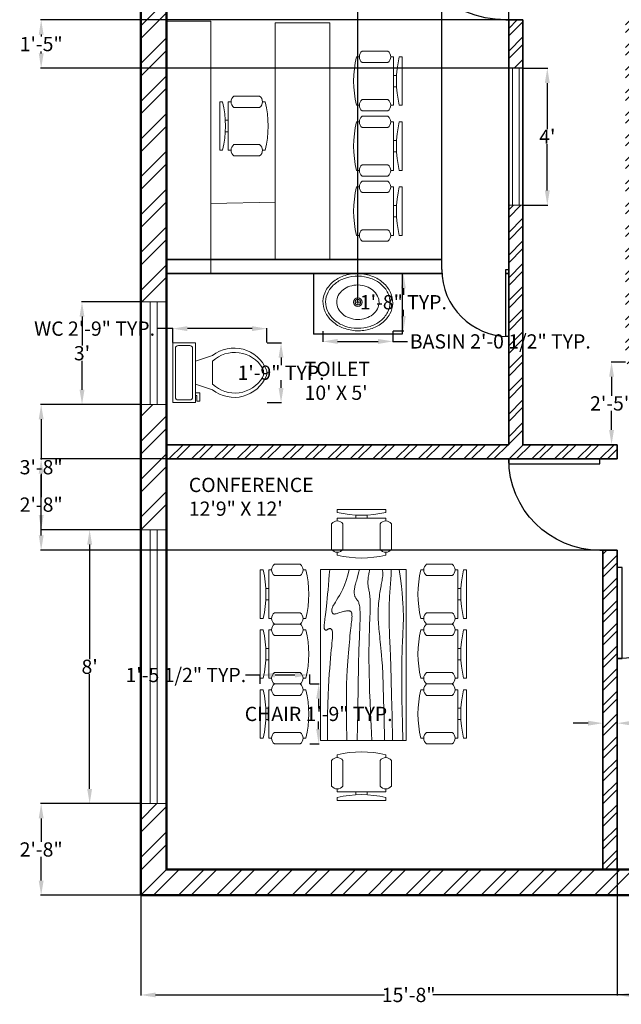
# Model space of a CAD drawing. Units: inches. Extents: x -355 to 263, y -871 to -163.
# Tile 1 of 6: x -344 to -133, y -867 to -521. Entities that reach past the tile are written whole.
import ezdxf

# ---------------------------------------------------------------- set-up
doc = ezdxf.new("R2010")
doc.units = ezdxf.units.IN
doc.header["$MEASUREMENT"] = 0
doc.layers.get('Defpoints').update_dxf_attribs({"color": 50})
for name, color, linetype, lineweight in [('A-ANNO-DIMS', 2, 'Continuous', 18), ('A-AREA-IDEN', 7, 'Continuous', 18), ('A-FLOR-CASE', 9, 'Continuous', 25), ('A-FLOR-FIXT', 8, 'Continuous', 18), ('A-WALL-PATT', 252, 'Continuous', 13)]:
    doc.layers.add(name, color=color, linetype=linetype, lineweight=lineweight)
for name, color, linetype, lineweight, plot in [('CHAIR', 8, 'Continuous', 18, False), ('DOOR', 4, 'Continuous', 25, False), ('IWAL', 7, 'Continuous', 35, False), ('OWALL', 7, 'Continuous', 50, False), ('TABLE', 8, 'Continuous', 18, False), ('WIND', 3, 'Continuous', 18, False)]:
    doc.layers.add(name, color=color, linetype=linetype, lineweight=lineweight, plot=plot)
doc.styles.get("Standard").update_dxf_attribs({"font": 'arial.ttf'})
doc.dimstyles.get("Standard").update_dxf_attribs({"dimtxt": 5, "dimasz": 5.18, "dimexe": 0.18, "dimexo": 0.0625, "dimgap": 0.09, "dimtad": 0, "dimtih": 1, "dimtoh": 1, "dimdec": 0, "dimzin": 0, "dimdsep": 46, "dimlunit": 3, "dimtxsty": 'Standard', "dimcen": 0.09, "dimadec": 0, "dimazin": 0, "dimtfac": 1, "dimtdec": 0, "dimtofl": 0, "dimtmove": 0, "dimatfit": 3, "dimfxl": 1, "dimtolj": 1, "dimtzin": 0, "dimarcsym": 0})

# ---------------------------------------------------------------- blocks, each defined once
blk = doc.blocks.new('*U6')
for p, q in [((0, 0), (0, -6)), ((32, 0), (32, -6))]:
    blk.add_line(p, q)
blk.add_lwpolyline([(0, 0), (0, 32), (1.75, 32), (1.75, 0)], close=True)
blk.add_arc((0, 0), 32, 0, 90)
blk = doc.blocks.new('*U5')
for p, q in [((0, 0), (0, -6)), ((40, 0), (40, -6))]:
    blk.add_line(p, q)
blk.add_lwpolyline([(0, 0), (0, 40), (1.75, 40), (1.75, 0)], close=True)
blk.add_arc((0, 0), 40, 0, 90)
blk = doc.blocks.new('*U7')
for p, q in [((0, 0), (0, -6)), ((36, 0), (36, -6))]:
    blk.add_line(p, q)
blk.add_lwpolyline([(0, 0), (0, 36), (1.75, 36), (1.75, 0)], close=True)
blk.add_arc((0, 0), 36, 0, 90)
blk = doc.blocks.new('Table - Rectangular Woodgrain 60 x 30 in.')
for p, q in [((0, 0), (0, -30)), ((60, 0), (0, 0)), ((60, -30), (60, 0)), ((0, -30), (60, -30))]:
    blk.add_line(p, q)
for points in [[(0, -2.4), (4.8155, -2.418), (9.0302, -2.4688), (12.709, -2.5477), (15.9167, -2.65), (18.7181, -2.7711), (21.1781, -2.9063), (23.3616, -3.0508), (25.3333, -3.2), (27.1477, -3.3495), (28.8172, -3.4958), (30.3437, -3.636), (31.7291, -3.7667), (32.9756, -3.8849), (34.0849, -3.9875), (35.059, -4.0714), (35.9, -4.1334), (36.6114, -4.1711), (37.2041, -4.1854), (37.6906, -4.1779), (38.0833, -4.15), (38.3948, -4.1034), (38.6375, -4.0396), (38.8239, -3.9602), (38.9666, -3.8667), (39.0764, -3.7608), (39.1573, -3.6448), (39.2116, -3.521), (39.2416, -3.3917), (39.2498, -3.2593), (39.2385, -3.1261), (39.21, -2.9944), (39.1666, -2.8667), (39.111, -2.7447), (39.0468, -2.6281), (38.978, -2.5163), (38.9083, -2.4083), (38.8418, -2.3035), (38.7823, -2.201), (38.7337, -2.1001), (38.7, -2), (38.6844, -1.9003), (38.6875, -1.8021), (38.7094, -1.707), (38.75, -1.6167), (38.8094, -1.5326), (38.8875, -1.4563), (38.9844, -1.3893), (39.1, -1.3333), (39.2351, -1.2896), (39.3937, -1.2583), (39.5804, -1.2396), (39.8, -1.2333), (40.057, -1.2396), (40.3562, -1.2583), (40.7023, -1.2896), (41.1, -1.3333), (41.5547, -1.3895), (42.0755, -1.4573), (42.6721, -1.5361), (43.3542, -1.625), (44.1316, -1.7233), (45.014, -1.8302), (46.0114, -1.9449), (47.1333, -2.0667), (48.3862, -2.1947), (49.7625, -2.3281), (51.2513, -2.4663), (52.8416, -2.6083), (54.5226, -2.7535), (56.2833, -2.9011), (58.1127, -3.0501), (60, -3.2)], [(0, -9.2), (6.5759, -9.0858), (11.9385, -9.0365), (16.2527, -9.0418), (19.6833, -9.0917), (22.3952, -9.1759), (24.5531, -9.2844), (26.322, -9.4069), (27.8666, -9.5333), (29.3241, -9.6553), (30.7203, -9.7719), (32.0532, -9.8837), (33.3208, -9.9917), (34.5213, -10.0965), (35.6526, -10.199), (36.7128, -10.2999), (37.7, -10.4), (38.6129, -10.4996), (39.4531, -10.5969), (40.223, -10.6895), (40.925, -10.775), (41.5613, -10.8512), (42.1344, -10.9156), (42.6465, -10.966), (43.1, -11), (43.4976, -11.0158), (43.8437, -11.0136), (44.143, -10.9942), (44.4, -10.9583), (44.6195, -10.9069), (44.8062, -10.8406), (44.9648, -10.7603), (45.1, -10.6667), (45.2155, -10.5598), (45.3114, -10.4365), (45.3871, -10.2929), (45.4416, -10.125), (45.4743, -9.929), (45.4844, -9.7011), (45.4709, -9.4371), (45.4333, -9.1333), (45.3716, -8.7883), (45.2896, -8.4104), (45.1919, -8.0107), (45.0833, -7.6), (44.9685, -7.1893), (44.8521, -6.7896), (44.7388, -6.4117), (44.6333, -6.0667), (44.54, -5.7628), (44.4614, -5.4979), (44.4001, -5.2675), (44.3583, -5.0667), (44.3384, -4.8909), (44.3427, -4.7354), (44.3736, -4.5956), (44.4333, -4.4667), (44.5236, -4.3453), (44.6427, -4.2333), (44.7884, -4.1339), (44.9583, -4.05), (45.1501, -3.9849), (45.3614, -3.9417), (45.59, -3.9234), (45.8333, -3.9333), (46.0915, -3.9749), (46.3734, -4.0531), (46.6906, -4.1736), (47.0542, -4.3417), (47.4756, -4.5629), (47.9661, -4.8427), (48.5372, -5.1866), (49.2, -5.6), (49.9676, -6.0844), (50.8594, -6.625), (51.8965, -7.2031), (53.1, -7.8), (54.491, -8.3969), (56.0906, -8.975), (57.9199, -9.5156), (60, -10)], [(0, -12.8), (5.1847, -12.9322), (9.6213, -13.0323), (13.3963, -13.1059), (16.5958, -13.1583), (19.3063, -13.1952), (21.614, -13.2219), (23.6054, -13.2439), (25.3666, -13.2667), (26.9728, -13.2947), (28.4531, -13.3281), (29.8256, -13.3663), (31.1083, -13.4083), (32.3191, -13.4535), (33.476, -13.501), (34.597, -13.5501), (35.7, -13.6), (36.7984, -13.6497), (37.8875, -13.6979), (38.9578, -13.743), (40, -13.7833), (41.0047, -13.8174), (41.9625, -13.8438), (42.864, -13.8607), (43.7, -13.8667), (44.4631, -13.8604), (45.1552, -13.8417), (45.7801, -13.8104), (46.3416, -13.7667), (46.8439, -13.7104), (47.2906, -13.6417), (47.6858, -13.5604), (48.0333, -13.4667), (48.3375, -13.3608), (48.6042, -13.2448), (48.8396, -13.121), (49.05, -12.9917), (49.2417, -12.8593), (49.4208, -12.7261), (49.5937, -12.5944), (49.7667, -12.4667), (49.9452, -12.3451), (50.1323, -12.2313), (50.3303, -12.1268), (50.5416, -12.0333), (50.7686, -11.9524), (51.0135, -11.8854), (51.2788, -11.8341), (51.5666, -11.8), (51.8785, -11.7843), (52.2116, -11.7865), (52.562, -11.8059), (52.926, -11.8417), (53.2998, -11.8931), (53.6795, -11.9594), (54.0614, -12.0397), (54.4416, -12.1333), (54.8223, -12.2401), (55.2293, -12.3625), (55.6942, -12.5037), (56.2489, -12.6667), (56.9251, -12.8547), (57.7545, -13.0708), (58.7689, -13.3182), (60, -13.6)], [(0, -18), (5.124, -17.7273), (9.6609, -17.5057), (13.6705, -17.3303), (17.2125, -17.1958), (20.3467, -17.0973), (23.1328, -17.0297), (25.6307, -16.9878), (27.9, -16.9667), (29.9928, -16.9617), (31.9302, -16.9703), (33.7254, -16.9907), (35.3917, -17.0208), (36.9423, -17.0588), (38.3906, -17.1026), (39.7499, -17.1503), (41.0333, -17.2), (42.2519, -17.2496), (43.4073, -17.2969), (44.4986, -17.3395), (45.525, -17.375), (46.4858, -17.4012), (47.3802, -17.4156), (48.2074, -17.416), (48.9667, -17.4), (49.6583, -17.3662), (50.2872, -17.3167), (50.8595, -17.2547), (51.3812, -17.1833), (51.8584, -17.1057), (52.2971, -17.025), (52.7034, -16.9443), (53.0833, -16.8667), (53.443, -16.7951), (53.789, -16.7313), (54.128, -16.6768), (54.4666, -16.6334), (54.8115, -16.6024), (55.1693, -16.5854), (55.5465, -16.5841), (55.95, -16.6), (56.3828, -16.6337), (56.8346, -16.6823), (57.2915, -16.7418), (57.7396, -16.8084), (58.165, -16.878), (58.5539, -16.9469), (58.8924, -17.0111), (59.1666, -17.0667), (59.3679, -17.1107), (59.5078, -17.1438), (59.6032, -17.1675), (59.6708, -17.1833), (59.7275, -17.193), (59.7901, -17.1979), (59.8753, -17.1998), (60, -17.2)], [(0, -22.4), (8.0098, -22.2501), (14.4094, -22.1011), (19.4168, -21.9535), (23.25, -21.8083), (26.1269, -21.6663), (28.2656, -21.5281), (29.884, -21.3947), (31.2, -21.2667), (32.3967, -21.1448), (33.5172, -21.0292), (34.5697, -20.9198), (35.5625, -20.8167), (36.5037, -20.7198), (37.4015, -20.6292), (38.2642, -20.5448), (39.1, -20.4667), (39.9164, -20.3951), (40.7187, -20.3313), (41.5117, -20.2768), (42.3, -20.2333), (43.0883, -20.2024), (43.8812, -20.1854), (44.6836, -20.1841), (45.5, -20.2), (46.3328, -20.234), (47.1747, -20.2844), (48.0163, -20.3488), (48.8479, -20.425), (49.66, -20.5106), (50.4429, -20.6031), (51.1872, -20.7004), (51.8833, -20.8), (52.5246, -20.8999), (53.1166, -20.9995), (53.6681, -21.0983), (54.1875, -21.1958), (54.6834, -21.2919), (55.1646, -21.3859), (55.6394, -21.4777), (56.1167, -21.5667), (56.6028, -21.6515), (57.0961, -21.7266), (57.5929, -21.7852), (58.0896, -21.8208), (58.5823, -21.8268), (59.0674, -21.7964), (59.5412, -21.723), (60, -21.6)], [(0, -25.2), (8.6355, -25.0504), (15.7026, -24.9031), (21.4049, -24.7606), (25.9458, -24.625), (29.529, -24.4988), (32.3578, -24.3844), (34.6359, -24.284), (36.5667, -24.2), (38.3213, -24.1341), (39.9417, -24.0854), (41.437, -24.0523), (42.8167, -24.0333), (44.0901, -24.0268), (45.2667, -24.0313), (46.3557, -24.0451), (47.3667, -24.0667), (48.309, -24.0947), (49.1928, -24.1287), (50.0284, -24.168), (50.826, -24.2125), (51.5959, -24.2617), (52.3483, -24.3151), (53.0935, -24.3725), (53.8417, -24.4334), (54.6009, -24.497), (55.3699, -24.561), (56.1454, -24.6226), (56.9239, -24.6792), (57.7021, -24.7279), (58.4764, -24.7662), (59.2435, -24.7911), (60, -24.8)], [(0, -28.8), (5.6867, -28.6681), (10.45, -28.5698), (14.407, -28.5012), (17.675, -28.4584), (20.3711, -28.4374), (22.6125, -28.4344), (24.5164, -28.4455), (26.2, -28.4667), (27.762, -28.4947), (29.2276, -28.5281), (30.6033, -28.5663), (31.8958, -28.6084), (33.1118, -28.6535), (34.2578, -28.7011), (35.3405, -28.7501), (36.3666, -28.8), (37.3443, -28.8497), (38.288, -28.8974), (39.2137, -28.9412), (40.1375, -28.9792), (41.0753, -29.0093), (42.0432, -29.0297), (43.0572, -29.0384), (44.1333, -29.0333), (45.2936, -29.0114), (46.5843, -28.9641), (48.0579, -28.8816), (49.7666, -28.7542), (51.7629, -28.5721), (54.0989, -28.3255), (56.8272, -28.0048), (60, -27.6)]]:
    blk.add_lwpolyline(points)
blk = doc.blocks.new('Chair - Desk')
for p, q in [((-8.5, 0), (-8.5, -1)), ((-8.5, 0), (8.5, 0)), ((8.5, 0), (8.5, -1)), ((-8.5, -3), (-8.5, -4)), ((-8.5, -3), (8.5, -3)), ((-2, -3), (-2, -1.9355)), ((2, -1.9576), (2, -3)), ((8.5, -3), (8.5, -4)), ((-10.5, -5), (-10.5, -14)), ((-6.5, -14), (-6.5, -5)), ((6.5, -5), (6.5, -14)), ((10.5, -14), (10.5, -5)), ((-8.5, -15), (-8.5, -16)), ((8.5, -15), (8.5, -16))]:
    blk.add_line(p, q)
for centre, radius, start, end in [((0, 34.625), 36.625, 256.5803, 283.4197), ((-8.5, -6.5), 2.5, 36.8699, 143.1301), ((8.5, -6.5), 2.5, 36.8699, 143.1301), ((-8.5, -12.5), 2.5, 216.8699, 323.1301), ((0, 19.625), 36.625, 256.5803, 283.4197), ((8.5, -12.5), 2.5, 216.8699, 323.1301)]:
    blk.add_arc(centre, radius, start, end)
blk = doc.blocks.new('Toilet - top')
for p, q in [((9.5, -6), (9.5, -2)), ((-10, -8.5), (-8, -8.5)), ((-10, -9.5), (-10, -8.5)), ((-7, -9.5), (-10, -9.5)), ((-8, -8.5), (-8, -8)), ((-7, -8), (-7, -9.5)), ((-4, -8), (-6, -14)), ((4, -8), (6, -14)), ((4, -14), (-4, -14))]:
    blk.add_line(p, q)
blk.add_lwpolyline([(10.5, -8), (10.5, 0), (-10.5, 0), (-10.5, -8)], close=True)
for points in [[(-9.5, -2), (-9.5, -6)], [(8.5, -1), (-8.5, -1)], [(-8.5, -7), (8.5, -7)]]:
    blk.add_lwpolyline(points)
for centre, radius, start, end in [((-8.62, -1.88), 0.884, 81.8699, 188.1301), ((8.62, -1.88), 0.884, 351.8699, 98.1301), ((-8.62, -6.12), 0.884, 171.8699, 278.1301), ((8.62, -6.12), 0.884, 261.8699, 8.1301), ((3.52, -21.58), 12.17, 141.4691, 247.9714), ((4.2, -21.82), 11.33, 136.3677, 238.9468), ((-3.52, -21.58), 12.17, 292.0284, 38.5307), ((-4.2, -21.82), 11.33, 301.053, 43.6321), ((0, -27.88), 4, 245.7318, 294.2682), ((0, -29), 4, 254.8605, 285.1395)]:
    blk.add_arc(centre, radius, start, end)
blk = doc.blocks.new('Sink - Oval top')
for p, q in [((-1, 0), (1, 0)), ((0, 1), (0, -1))]:
    blk.add_line(p, q)
for points in [[(-12.23, 0.39, 0.117634), (-11.46, -3.36, 0.104469), (-8.88, -6.8, 0.090016), (-5.08, -9.07, 0.08192), (-0.32, -10.02, 0.08192), (4.49, -9.38, 0.090016), (8.42, -7.36, 0.104469), (11.22, -4.09, 0.117634), (12.23, -0.39, 0.117634), (11.46, 3.36, 0.104469), (8.88, 6.8, 0.090016), (5.08, 9.07, 0.08192), (0.32, 10.02, 0.08192), (-4.49, 9.38, 0.090016), (-8.42, 7.36, 0.104469), (-11.22, 4.09, 0.117634)], [(-11.29, 0.16, 0.118622), (-10.52, -3.25, 0.104678), (-8.07, -6.36, 0.089562), (-4.54, -8.37, 0.081185), (-0.13, -9.15, 0.081185), (4.3, -8.49, 0.089562), (7.89, -6.58, 0.104678), (10.42, -3.55, 0.118622), (11.29, -0.16, 0.118622), (10.52, 3.25, 0.104678), (8.07, 6.36, 0.089562), (4.54, 8.37, 0.081185), (0.13, 9.15, 0.081185), (-4.3, 8.49, 0.089562), (-7.89, 6.58, 0.104678), (-10.42, 3.55, 0.118622)], [(-7.42, 0.08, 0.118283), (-6.91, -2.17, 0.104607), (-5.29, -4.21, 0.089718), (-2.97, -5.53, 0.081436), (-0.07, -6.04, 0.081436), (2.84, -5.59, 0.089718), (5.2, -4.33, 0.104607), (6.86, -2.32, 0.118283), (7.42, -0.08, 0.118283), (6.91, 2.17, 0.104607), (5.29, 4.21, 0.089718), (2.97, 5.53, 0.081436), (0.07, 6.04, 0.081436), (-2.84, 5.59, 0.089718), (-5.2, 4.33, 0.104607), (-6.86, 2.32, 0.118283)]]:
    blk.add_lwpolyline(points, format="xyb", close=True)
for radius in [1.5, 1]:
    blk.add_circle((0, 0), radius)
blk = doc.blocks.new('*D48')
at = {"layer": 'A-ANNO-DIMS', "color": 0, "lineweight": -2, "transparency": 16777216}
for p, q in [((-139.32, -763.34), (-139.32, -768.11)), ((-134.32, -763.34), (-134.32, -768.11)), ((-144.5, -767.93), (-149.68, -767.93)), ((-129.14, -767.93), (-123.96, -767.93))]:
    blk.add_line(p, q, dxfattribs=at)
at = {"layer": 'A-ANNO-DIMS', "color": 0, "lineweight": -3, "transparency": 16777216}
for points in [[(-144.5, -767.07), (-144.5, -768.79), (-139.32, -767.93)], [(-129.14, -767.07), (-129.14, -768.79), (-134.32, -767.93)]]:
    blk.add_solid(points, dxfattribs=at)
at = {"layer": 'Defpoints', "color": 0, "lineweight": -3, "transparency": 16777216}
for p in [(-139.32, -763.28), (-134.32, -763.28), (-134.32, -767.93)]:
    blk.add_point(p, dxfattribs=at)
at = {"layer": 'A-ANNO-DIMS', "color": 0, "transparency": 16777216, "insert": (-121, -767.93), "char_height": 5, "attachment_point": 5}
blk.add_mtext('\\A1;5"', dxfattribs=at)
blk = doc.blocks.new('*D49')
at = {"layer": 'A-ANNO-DIMS', "color": 0, "lineweight": -2, "transparency": 16777216}
for p, q in [((-301.38, -700.14), (-319.45, -700.14)), ((-319.27, -705.32), (-319.27, -745.49)), ((-319.27, -790.96), (-319.27, -750.78)), ((-301.38, -796.14), (-319.45, -796.14))]:
    blk.add_line(p, q, dxfattribs=at)
at = {"layer": 'A-ANNO-DIMS', "color": 0, "lineweight": -3, "transparency": 16777216}
for points in [[(-320.14, -705.32), (-318.41, -705.32), (-319.27, -700.14)], [(-320.14, -790.96), (-318.41, -790.96), (-319.27, -796.14)]]:
    blk.add_solid(points, dxfattribs=at)
at = {"layer": 'Defpoints', "color": 0, "lineweight": -3, "transparency": 16777216}
for p in [(-319.27, -700.14), (-301.32, -700.14), (-301.32, -796.14)]:
    blk.add_point(p, dxfattribs=at)
at = {"layer": 'A-ANNO-DIMS', "color": 0, "transparency": 16777216, "insert": (-319.27, -748.14), "char_height": 5, "attachment_point": 5}
blk.add_mtext("\\A1;8'", dxfattribs=at)
blk = doc.blocks.new('*D50')
at = {"layer": 'A-ANNO-DIMS', "color": 0, "lineweight": -2, "transparency": 16777216}
for p, q in [((-301.38, -620.18), (-322.13, -620.18)), ((-321.95, -625.36), (-321.95, -635.53)), ((-321.95, -651), (-321.95, -640.82)), ((-301.38, -656.18), (-322.13, -656.18))]:
    blk.add_line(p, q, dxfattribs=at)
at = {"layer": 'A-ANNO-DIMS', "color": 0, "lineweight": -3, "transparency": 16777216}
for points in [[(-322.81, -625.36), (-321.09, -625.36), (-321.95, -620.18)], [(-322.81, -651), (-321.09, -651), (-321.95, -656.18)]]:
    blk.add_solid(points, dxfattribs=at)
at = {"layer": 'Defpoints', "color": 0, "lineweight": -3, "transparency": 16777216}
for p in [(-321.95, -620.18), (-301.32, -620.18), (-301.32, -656.18)]:
    blk.add_point(p, dxfattribs=at)
at = {"layer": 'A-ANNO-DIMS', "color": 0, "transparency": 16777216, "insert": (-321.95, -638.18), "char_height": 5, "attachment_point": 5}
blk.add_mtext("\\A1;3'", dxfattribs=at)
blk = doc.blocks.new('*D52')
at = {"layer": 'A-ANNO-DIMS', "color": 0, "lineweight": -2, "transparency": 16777216}
for p, q in [((-167.26, -538.25), (-158.59, -538.25)), ((-158.77, -543.43), (-158.77, -559.66)), ((-158.77, -581.07), (-158.77, -564.84)), ((-167.26, -586.25), (-158.59, -586.25))]:
    blk.add_line(p, q, dxfattribs=at)
at = {"layer": 'A-ANNO-DIMS', "color": 0, "lineweight": -3, "transparency": 16777216}
for points in [[(-159.64, -543.43), (-157.91, -543.43), (-158.77, -538.25)], [(-159.64, -581.07), (-157.91, -581.07), (-158.77, -586.25)]]:
    blk.add_solid(points, dxfattribs=at)
at = {"layer": 'Defpoints', "color": 0, "lineweight": -3, "transparency": 16777216}
for p in [(-167.32, -538.25), (-158.77, -538.25), (-167.32, -586.25)]:
    blk.add_point(p, dxfattribs=at)
at = {"layer": 'A-ANNO-DIMS', "color": 0, "transparency": 16777216, "insert": (-158.77, -562.25), "char_height": 5, "attachment_point": 5}
blk.add_mtext("\\A1;4'", dxfattribs=at)
blk = doc.blocks.new('*D53')
at = {"layer": 'A-ANNO-DIMS', "color": 0, "lineweight": -2, "transparency": 16777216}
for p, q in [((-131.38, -641.28), (-136.42, -641.28)), ((-136.24, -646.46), (-136.24, -653.14)), ((-136.24, -665.1), (-136.24, -658.42)), ((-134.38, -670.28), (-136.42, -670.28))]:
    blk.add_line(p, q, dxfattribs=at)
at = {"layer": 'A-ANNO-DIMS', "color": 0, "lineweight": -3, "transparency": 16777216}
for points in [[(-137.1, -646.46), (-135.38, -646.46), (-136.24, -641.28)], [(-137.1, -665.1), (-135.38, -665.1), (-136.24, -670.28)]]:
    blk.add_solid(points, dxfattribs=at)
at = {"layer": 'Defpoints', "color": 0, "lineweight": -3, "transparency": 16777216}
for p in [(-136.24, -641.28), (-131.32, -641.28), (-134.32, -670.28)]:
    blk.add_point(p, dxfattribs=at)
at = {"layer": 'A-ANNO-DIMS', "color": 0, "transparency": 16777216, "insert": (-136.24, -655.78), "char_height": 5, "attachment_point": 5}
blk.add_mtext('\\A1;2\'-5"', dxfattribs=at)
blk = doc.blocks.new('WIN-36IN-9IN-WALL')
for p, q in [((4.5, 36), (0, 36)), ((3.3, 36), (3.3, 0)), ((4.5, 36), (9, 36)), ((5.7, 36), (5.7, 0)), ((4.5, 0), (0, 0)), ((4.5, 0), (9, 0))]:
    blk.add_line(p, q)
blk = doc.blocks.new('WIN-48IN-5IN-WALL')
for p, q in [((2.5, 48), (0, 48)), ((1.3, 48), (1.3, 0)), ((2.5, 48), (5, 48)), ((3.7, 48), (3.7, 0)), ((2.5, 0), (0, 0)), ((2.5, 0), (5, 0))]:
    blk.add_line(p, q)
blk = doc.blocks.new('*D61')
at = {"layer": 'A-ANNO-DIMS', "color": 0, "lineweight": -2, "transparency": 16777216}
for p, q in [((-242.05, -754.18), (-238.78, -754.18)), ((-238.96, -759.36), (-238.96, -762)), ((-238.96, -770), (-238.96, -767.35)), ((-242.05, -775.18), (-238.78, -775.18))]:
    blk.add_line(p, q, dxfattribs=at)
at = {"layer": 'A-ANNO-DIMS', "color": 0, "lineweight": -3, "transparency": 16777216}
for points in [[(-239.82, -759.36), (-238.1, -759.36), (-238.96, -754.18)], [(-239.82, -770), (-238.1, -770), (-238.96, -775.18)]]:
    blk.add_solid(points, dxfattribs=at)
at = {"layer": 'Defpoints', "color": 0, "lineweight": -3, "transparency": 16777216}
for p in [(-242.11, -754.18), (-238.96, -754.18), (-242.11, -775.18)]:
    blk.add_point(p, dxfattribs=at)
at = {"layer": 'A-ANNO-DIMS', "color": 0, "transparency": 16777216, "insert": (-238.96, -764.68), "char_height": 5, "attachment_point": 5}
blk.add_mtext('\\A1;CHAIR 1\'-9" TYP.', dxfattribs=at)
blk = doc.blocks.new('*D62')
at = {"layer": 'A-ANNO-DIMS', "color": 0, "lineweight": -2, "transparency": 16777216}
for p, q in [((-259.44, -751.03), (-264.62, -751.03)), ((-259.44, -754.11), (-259.44, -750.85)), ((-247.29, -751.03), (-254.26, -751.03)), ((-242.11, -754.11), (-242.11, -750.85))]:
    blk.add_line(p, q, dxfattribs=at)
at = {"layer": 'A-ANNO-DIMS', "color": 0, "lineweight": -3, "transparency": 16777216}
for points in [[(-254.26, -750.16), (-254.26, -751.89), (-259.44, -751.03)], [(-247.29, -750.16), (-247.29, -751.89), (-242.11, -751.03)]]:
    blk.add_solid(points, dxfattribs=at)
at = {"layer": 'Defpoints', "color": 0, "lineweight": -3, "transparency": 16777216}
for p in [(-259.44, -751.03), (-259.44, -754.18), (-242.11, -754.18)]:
    blk.add_point(p, dxfattribs=at)
at = {"layer": 'A-ANNO-DIMS', "color": 0, "transparency": 16777216, "insert": (-285.54, -751.03), "char_height": 5, "attachment_point": 5}
blk.add_mtext('\\A1;1\'-5 1/2" TYP.', dxfattribs=at)
blk = doc.blocks.new('*D63')
at = {"layer": 'A-ANNO-DIMS', "color": 0, "lineweight": -2, "transparency": 16777216}
for p, q in [((-290.15, -629.56), (-295.33, -629.56)), ((-290.15, -634.46), (-290.15, -629.38)), ((-262.29, -629.56), (-284.97, -629.56)), ((-257.11, -634.46), (-257.11, -629.38))]:
    blk.add_line(p, q, dxfattribs=at)
at = {"layer": 'A-ANNO-DIMS', "color": 0, "lineweight": -3, "transparency": 16777216}
for points in [[(-284.97, -628.7), (-284.97, -630.43), (-290.15, -629.56)], [(-262.29, -628.7), (-262.29, -630.43), (-257.11, -629.56)]]:
    blk.add_solid(points, dxfattribs=at)
at = {"layer": 'Defpoints', "color": 0, "lineweight": -3, "transparency": 16777216}
for p in [(-290.15, -629.56), (-290.15, -634.52), (-257.11, -634.52)]:
    blk.add_point(p, dxfattribs=at)
at = {"layer": 'A-ANNO-DIMS', "color": 0, "transparency": 16777216, "insert": (-317.55, -629.56), "char_height": 5, "attachment_point": 5}
blk.add_mtext('\\A1;WC 2\'-9" TYP.', dxfattribs=at)
blk = doc.blocks.new('*D64')
at = {"layer": 'A-ANNO-DIMS', "color": 0, "lineweight": -2, "transparency": 16777216}
for p, q in [((-257.05, -634.52), (-251.97, -634.52)), ((-252.15, -639.7), (-252.15, -642.38)), ((-252.15, -650.34), (-252.15, -647.66)), ((-257.05, -655.52), (-251.97, -655.52))]:
    blk.add_line(p, q, dxfattribs=at)
at = {"layer": 'A-ANNO-DIMS', "color": 0, "lineweight": -3, "transparency": 16777216}
for points in [[(-253.01, -639.7), (-251.29, -639.7), (-252.15, -634.52)], [(-253.01, -650.34), (-251.29, -650.34), (-252.15, -655.52)]]:
    blk.add_solid(points, dxfattribs=at)
at = {"layer": 'Defpoints', "color": 0, "lineweight": -3, "transparency": 16777216}
for p in [(-257.11, -634.52), (-252.15, -634.52), (-257.11, -655.52)]:
    blk.add_point(p, dxfattribs=at)
at = {"layer": 'A-ANNO-DIMS', "color": 0, "transparency": 16777216, "insert": (-252.15, -645.02), "char_height": 5, "attachment_point": 5}
blk.add_mtext('\\A1;1\'-9" TYP.', dxfattribs=at)
blk = doc.blocks.new('*D65')
at = {"layer": 'A-ANNO-DIMS', "color": 0, "lineweight": -2, "transparency": 16777216}
for p, q in [((-237.48, -630.43), (-237.48, -634.23)), ((-212.93, -630.43), (-212.93, -634.23)), ((-232.3, -634.05), (-218.11, -634.05)), ((-212.93, -634.05), (-207.75, -634.05))]:
    blk.add_line(p, q, dxfattribs=at)
at = {"layer": 'A-ANNO-DIMS', "color": 0, "lineweight": -3, "transparency": 16777216}
for points in [[(-232.3, -633.19), (-232.3, -634.92), (-237.48, -634.05)], [(-218.11, -633.19), (-218.11, -634.92), (-212.93, -634.05)]]:
    blk.add_solid(points, dxfattribs=at)
at = {"layer": 'Defpoints', "color": 0, "lineweight": -3, "transparency": 16777216}
for p in [(-237.48, -630.37), (-212.93, -630.37), (-212.93, -634.05)]:
    blk.add_point(p, dxfattribs=at)
at = {"layer": 'A-ANNO-DIMS', "color": 0, "transparency": 16777216, "insert": (-175.26, -634.05), "char_height": 5, "attachment_point": 5}
blk.add_mtext('\\A1;BASIN 2\'-0 1/2" TYP.', dxfattribs=at)
blk = doc.blocks.new('*D66')
at = {"layer": 'A-ANNO-DIMS', "color": 0, "lineweight": -2, "transparency": 16777216}
for p, q in [((-212.87, -610.24), (-209.07, -610.24)), ((-209.25, -615.42), (-209.25, -617.66)), ((-209.25, -625.19), (-209.25, -622.95)), ((-212.87, -630.37), (-209.07, -630.37))]:
    blk.add_line(p, q, dxfattribs=at)
at = {"layer": 'A-ANNO-DIMS', "color": 0, "lineweight": -3, "transparency": 16777216}
for points in [[(-210.11, -615.42), (-208.39, -615.42), (-209.25, -610.24)], [(-210.11, -625.19), (-208.39, -625.19), (-209.25, -630.37)]]:
    blk.add_solid(points, dxfattribs=at)
at = {"layer": 'Defpoints', "color": 0, "lineweight": -3, "transparency": 16777216}
for p in [(-212.93, -610.24), (-209.25, -610.24), (-212.93, -630.37)]:
    blk.add_point(p, dxfattribs=at)
at = {"layer": 'A-ANNO-DIMS', "color": 0, "transparency": 16777216, "insert": (-209.25, -620.3), "char_height": 5, "attachment_point": 5}
blk.add_mtext('\\A1;1\'-8" TYP.', dxfattribs=at)
blk = doc.blocks.new('*D79')
at = {"layer": 'A-ANNO-DIMS', "color": 0, "lineweight": -2, "transparency": 16777216}
for p, q in [((-301.38, -796.14), (-336.45, -796.14)), ((-336.27, -801.32), (-336.27, -809.57)), ((-336.27, -823.1), (-336.27, -814.85)), ((-301.38, -828.28), (-336.45, -828.28))]:
    blk.add_line(p, q, dxfattribs=at)
at = {"layer": 'A-ANNO-DIMS', "color": 0, "lineweight": -3, "transparency": 16777216}
for points in [[(-337.13, -801.32), (-335.41, -801.32), (-336.27, -796.14)], [(-337.13, -823.1), (-335.41, -823.1), (-336.27, -828.28)]]:
    blk.add_solid(points, dxfattribs=at)
at = {"layer": 'Defpoints', "color": 0, "lineweight": -3, "transparency": 16777216}
for p in [(-336.27, -796.14), (-301.32, -796.14), (-301.32, -828.28)]:
    blk.add_point(p, dxfattribs=at)
at = {"layer": 'A-ANNO-DIMS', "color": 0, "transparency": 16777216, "insert": (-336.27, -812.21), "char_height": 5, "attachment_point": 5}
blk.add_mtext('\\A1;2\'-8"', dxfattribs=at)
blk = doc.blocks.new('*D80')
at = {"layer": 'A-ANNO-DIMS', "color": 0, "lineweight": -2, "transparency": 16777216}
for p, q in [((-301.38, -656.18), (-336.45, -656.18)), ((-336.27, -661.36), (-336.27, -675.51)), ((-336.27, -694.96), (-336.27, -680.8)), ((-301.38, -700.14), (-336.45, -700.14))]:
    blk.add_line(p, q, dxfattribs=at)
at = {"layer": 'A-ANNO-DIMS', "color": 0, "lineweight": -3, "transparency": 16777216}
for points in [[(-337.13, -661.36), (-335.41, -661.36), (-336.27, -656.18)], [(-337.13, -694.96), (-335.41, -694.96), (-336.27, -700.14)]]:
    blk.add_solid(points, dxfattribs=at)
at = {"layer": 'Defpoints', "color": 0, "lineweight": -3, "transparency": 16777216}
for p in [(-336.27, -656.18), (-301.32, -656.18), (-301.32, -700.14)]:
    blk.add_point(p, dxfattribs=at)
at = {"layer": 'A-ANNO-DIMS', "color": 0, "transparency": 16777216, "insert": (-336.27, -678.16), "char_height": 5, "attachment_point": 5}
blk.add_mtext('\\A1;3\'-8"', dxfattribs=at)
blk = doc.blocks.new('*D82')
at = {"layer": 'A-ANNO-DIMS', "color": 0, "lineweight": -2, "transparency": 16777216}
for p, q in [((-301.32, -828.34), (-301.32, -863.41)), ((-113.45, -828.34), (-113.45, -863.41)), ((-296.14, -863.23), (-215.83, -863.23)), ((-118.63, -863.23), (-198.94, -863.23))]:
    blk.add_line(p, q, dxfattribs=at)
at = {"layer": 'A-ANNO-DIMS', "color": 0, "lineweight": -3, "transparency": 16777216}
for points in [[(-296.14, -862.37), (-296.14, -864.09), (-301.32, -863.23)], [(-118.63, -862.37), (-118.63, -864.09), (-113.45, -863.23)]]:
    blk.add_solid(points, dxfattribs=at)
at = {"layer": 'Defpoints', "color": 0, "lineweight": -3, "transparency": 16777216}
for p in [(-301.32, -828.28), (-113.45, -828.28), (-113.45, -863.23)]:
    blk.add_point(p, dxfattribs=at)
at = {"layer": 'A-ANNO-DIMS', "color": 0, "transparency": 16777216, "insert": (-207.39, -863.23), "char_height": 5, "attachment_point": 5}
blk.add_mtext('\\A1;15\'-8"', dxfattribs=at)
blk = doc.blocks.new('*D84')
at = {"layer": 'A-ANNO-DIMS', "color": 0, "lineweight": -2, "transparency": 16777216}
for p, q in [((-195.8, -605.22), (-195.8, -181.15)), ((-190.62, -181.33), (-177.5, -181.33)), ((-172.32, -605.22), (-172.32, -181.15)), ((-172.32, -181.33), (-167.14, -181.33))]:
    blk.add_line(p, q, dxfattribs=at)
at = {"layer": 'A-ANNO-DIMS', "color": 0, "lineweight": -3, "transparency": 16777216}
for points in [[(-190.62, -180.47), (-190.62, -182.19), (-195.8, -181.33)], [(-177.5, -180.47), (-177.5, -182.19), (-172.32, -181.33)]]:
    blk.add_solid(points, dxfattribs=at)
at = {"layer": 'Defpoints', "color": 0, "lineweight": -3, "transparency": 16777216}
for p in [(-172.32, -181.33), (-195.8, -605.28), (-172.32, -605.28)]:
    blk.add_point(p, dxfattribs=at)
at = {"layer": 'A-ANNO-DIMS', "color": 0, "transparency": 16777216, "insert": (-152.87, -181.33), "char_height": 5, "attachment_point": 5}
blk.add_mtext('\\A1;1\'-11 1/2"', dxfattribs=at)
blk = doc.blocks.new('*D85')
at = {"layer": 'A-ANNO-DIMS', "color": 0, "lineweight": -2, "transparency": 16777216}
for p, q in [((-292.32, -610.22), (-292.32, -181.15)), ((-287.14, -181.33), (-265.5, -181.33)), ((-230.39, -181.33), (-252.03, -181.33)), ((-225.21, -620.24), (-225.21, -181.15))]:
    blk.add_line(p, q, dxfattribs=at)
at = {"layer": 'A-ANNO-DIMS', "color": 0, "lineweight": -3, "transparency": 16777216}
for points in [[(-287.14, -180.47), (-287.14, -182.19), (-292.32, -181.33)], [(-230.39, -180.47), (-230.39, -182.19), (-225.21, -181.33)]]:
    blk.add_solid(points, dxfattribs=at)
at = {"layer": 'Defpoints', "color": 0, "lineweight": -3, "transparency": 16777216}
for p in [(-225.21, -181.33), (-292.32, -610.28), (-225.21, -620.3)]:
    blk.add_point(p, dxfattribs=at)
at = {"layer": 'A-ANNO-DIMS', "color": 0, "transparency": 16777216, "insert": (-258.76, -181.33), "char_height": 5, "attachment_point": 5}
blk.add_mtext('\\A1;5\'-7"', dxfattribs=at)
blk = doc.blocks.new('*D87')
at = {"layer": 'A-ANNO-DIMS', "color": 0, "lineweight": -2, "transparency": 16777216}
for p, q in [((-134.38, -675.28), (-336.45, -675.28)), ((-336.27, -680.46), (-336.27, -688.64)), ((-336.27, -702.1), (-336.27, -693.92)), ((-134.38, -707.28), (-336.45, -707.28))]:
    blk.add_line(p, q, dxfattribs=at)
at = {"layer": 'A-ANNO-DIMS', "color": 0, "lineweight": -3, "transparency": 16777216}
for points in [[(-337.13, -680.46), (-335.41, -680.46), (-336.27, -675.28)], [(-337.13, -702.1), (-335.41, -702.1), (-336.27, -707.28)]]:
    blk.add_solid(points, dxfattribs=at)
at = {"layer": 'Defpoints', "color": 0, "lineweight": -3, "transparency": 16777216}
for p in [(-134.32, -675.28), (-336.27, -707.28), (-134.32, -707.28)]:
    blk.add_point(p, dxfattribs=at)
at = {"layer": 'A-ANNO-DIMS', "color": 0, "transparency": 16777216, "insert": (-336.27, -691.28), "char_height": 5, "attachment_point": 5}
blk.add_mtext('\\A1;2\'-8"', dxfattribs=at)
blk = doc.blocks.new('*D88')
at = {"layer": 'A-ANNO-DIMS', "color": 0, "lineweight": -2, "transparency": 16777216}
for p, q in [((-134.32, -707.34), (-134.32, -863.41)), ((-102.32, -707.34), (-102.32, -863.41)), ((-129.14, -863.23), (-125.1, -863.23)), ((-107.5, -863.23), (-111.54, -863.23))]:
    blk.add_line(p, q, dxfattribs=at)
at = {"layer": 'A-ANNO-DIMS', "color": 0, "lineweight": -3, "transparency": 16777216}
for points in [[(-129.14, -862.37), (-129.14, -864.09), (-134.32, -863.23)], [(-107.5, -862.37), (-107.5, -864.09), (-102.32, -863.23)]]:
    blk.add_solid(points, dxfattribs=at)
at = {"layer": 'Defpoints', "color": 0, "lineweight": -3, "transparency": 16777216}
for p in [(-134.32, -707.28), (-102.32, -707.28), (-102.32, -863.23)]:
    blk.add_point(p, dxfattribs=at)
at = {"layer": 'A-ANNO-DIMS', "color": 0, "transparency": 16777216, "insert": (-118.32, -863.23), "char_height": 5, "attachment_point": 5}
blk.add_mtext('\\A1;2\'-8"', dxfattribs=at)
blk = doc.blocks.new('*D94')
at = {"layer": 'A-ANNO-DIMS', "color": 0, "lineweight": -2, "transparency": 16777216}
for p, q in [((-167.38, -521.28), (-336.45, -521.28)), ((-336.27, -526.46), (-336.27, -527.12)), ((-336.27, -533.07), (-336.27, -532.41)), ((-167.38, -538.25), (-336.45, -538.25))]:
    blk.add_line(p, q, dxfattribs=at)
at = {"layer": 'A-ANNO-DIMS', "color": 0, "lineweight": -3, "transparency": 16777216}
for points in [[(-337.13, -526.46), (-335.41, -526.46), (-336.27, -521.28)], [(-337.13, -533.07), (-335.41, -533.07), (-336.27, -538.25)]]:
    blk.add_solid(points, dxfattribs=at)
at = {"layer": 'Defpoints', "color": 0, "lineweight": -3, "transparency": 16777216}
for p in [(-167.32, -521.28), (-336.27, -538.25), (-167.32, -538.25)]:
    blk.add_point(p, dxfattribs=at)
at = {"layer": 'A-ANNO-DIMS', "color": 0, "transparency": 16777216, "insert": (-336.27, -529.76), "char_height": 5, "attachment_point": 5}
blk.add_mtext('\\A1;1\'-5"', dxfattribs=at)

msp = doc.modelspace()

# ---------------------------------------------------------------- hatches: boundary and pattern name
at = {"layer": 'A-WALL-PATT'}
h = msp.add_hatch(dxfattribs=at)
h.set_pattern_fill('ANSI32', color=256, scale=25)
h.set_pattern_definition([(45, (-301.32, -828.28), (-6.62913, 6.62913), []), (45, (-296.9, -828.28), (-6.62913, 6.62913), [])])
h.paths.add_polyline_path([(54.68, -289.28), (-301.32, -289.28), (-301.32, -303.28), (-295.02, -303.28), (-292.32, -303.28), (-292.32, -298.28), (54.68, -298.28)])
h.paths.add_polyline_path([(188.68, -216.28), (54.68, -216.28), (54.68, -225.28), (179.68, -225.28), (179.68, -345.28), (179.68, -485.16), (184.18, -485.16), (188.68, -485.16)])
h.paths.add_polyline_path([(188.68, -521.16), (184.18, -521.16), (179.68, -521.16), (179.68, -540.28), (188.68, -540.28)])
h.paths.add_polyline_path([(164.68, -540.28), (155.68, -540.28), (155.68, -552.97), (160.18, -552.97), (164.68, -552.97)])
h.paths.add_polyline_path([(164.68, -588.97), (160.18, -588.97), (155.68, -588.97), (155.68, -620.04), (160.18, -620.04), (164.68, -620.04)])
h.paths.add_polyline_path([(164.68, -656.04), (160.18, -656.04), (155.68, -656.04), (155.68, -682.06), (160.18, -682.06), (164.68, -682.06)])
h.paths.add_polyline_path([(164.68, -718.06), (160.18, -718.06), (155.68, -718.06), (155.68, -730.28), (164.68, -730.28)])
h.paths.add_polyline_path([(188.68, -730.28), (179.68, -730.28), (179.68, -819.28), (73.9, -819.28), (73.9, -823.78), (73.9, -828.28), (188.68, -828.28)])
h.paths.add_polyline_path([(25.9, -819.28), (-41.45, -819.28), (-41.45, -823.78), (-41.45, -828.28), (25.9, -828.28), (25.9, -823.78)])
h.paths.add_polyline_path([(-113.45, -819.28), (-292.32, -819.28), (-292.32, -796.14), (-296.82, -796.14), (-301.32, -796.14), (-301.32, -828.28), (-113.45, -828.28), (-113.45, -823.78)])
h.paths.add_polyline_path([(-292.32, -480.28), (-292.32, -345.28), (-301.32, -345.28), (-301.32, -620.18), (-296.82, -620.18), (-292.32, -620.18)])
h.paths.add_polyline_path([(-292.32, -656.18), (-296.82, -656.18), (-301.32, -656.18), (-301.32, -700.14), (-296.82, -700.14), (-292.32, -700.14)])
h = msp.add_hatch(dxfattribs=at)
h.set_pattern_fill('ANSI32', color=256, scale=15)
h.set_pattern_definition([(45, (-292.3197, -819.28), (-3.977476, 3.977476), []), (45, (-289.668, -819.28), (-3.977476, 3.977476), [])])
h.paths.add_polyline_path([(59.68, -280.18), (57.18, -280.18), (54.68, -280.18), (54.68, -289.28), (54.68, -298.28), (54.68, -303.28), (59.68, -303.28)])
h.paths.add_polyline_path([(59.68, -225.28), (54.68, -225.28), (54.68, -232.18), (57.18, -232.18), (59.68, -232.18)])
h.paths.add_polyline_path([(18.68, -641.28), (18.68, -521.28), (13.68, -521.28), (13.68, -641.28), (-7.32, -665.28), (-105.32, -665.28), (-126.32, -641.28), (-126.32, -521.28), (-131.32, -521.28), (-131.32, -641.28), (-105.32, -670.28), (-7.32, -670.28)])
h.paths.add_polyline_path([(-167.32, -521.28), (-172.32, -521.28), (-172.32, -538.25), (-169.82, -538.25), (-167.32, -538.25)])
h.paths.add_polyline_path([(-134.32, -670.28), (-167.32, -670.28), (-167.32, -610.28), (-167.32, -586.25), (-169.82, -586.25), (-172.32, -586.25), (-172.32, -670.28), (-292.32, -670.28), (-292.32, -675.28), (-139.32, -675.28), (-134.32, -675.28)])
h.paths.add_polyline_path([(-167.32, -345.28), (-172.32, -345.28), (-172.32, -462.28), (-172.32, -480.28), (-292.32, -480.28), (-292.32, -485.28), (-172.32, -485.28), (-167.32, -485.28), (5.68, -485.28), (5.68, -480.28), (-167.32, -480.28)])
h.paths.add_polyline_path([(179.68, -345.28), (30.68, -345.28), (30.68, -365.65), (33.18, -365.65), (35.68, -365.65), (35.68, -350.28), (179.68, -350.28)])
h.paths.add_polyline_path([(-134.32, -707.28), (-139.32, -707.28), (-139.32, -819.28), (-134.32, -819.28)])
h.paths.add_polyline_path([(-9.32, -707.28), (-102.32, -707.28), (-102.32, -712.28), (-14.32, -712.28), (-14.32, -819.28), (-9.32, -819.28)])
h.paths.add_polyline_path([(179.68, -730.28), (22.68, -730.28), (22.68, -735.28), (179.68, -735.28)])
h.paths.add_polyline_path([(179.68, -470.28), (30.68, -470.28), (30.68, -475.28), (54.68, -475.28), (54.68, -505.29), (59.18, -505.29, -0.00418), (59.68, -505.29), (59.68, -475.28), (179.68, -475.28)])
h.paths.add_polyline_path([(35.68, -413.65), (33.18, -413.65), (30.68, -413.65), (30.68, -440.29), (35.18, -440.29, -0.00418), (35.68, -440.29)])
h.paths.add_polyline_path([(179.68, -535.28), (54.68, -535.28), (54.68, -540.28), (54.68, -570.29), (59.18, -570.29, -0.00418), (59.68, -570.29), (59.68, -540.28), (179.68, -540.28)])
h.paths.add_polyline_path([(121.93, -531.51), (160.73, -531.51), (160.73, -512.85), (121.93, -512.85)], flags=9)
h.paths.add_polyline_path([(49.47, -376.48), (111.2, -376.48), (111.2, -357.82), (49.47, -357.82)], flags=9)

# ---------------------------------------------------------------- linework, layer by layer
at = {"layer": 'A-FLOR-CASE'}
for p, q in [((-240.75, -610.28), (-240.75, -631.45)), ((-209.66, -610.28), (-209.66, -631.45)), ((-209.66, -631.45), (-240.75, -631.45))]:
    msp.add_line(p, q, dxfattribs=at)
at = {"layer": 'IWAL'}
for p, q in [((-172.32, -670.28), (-172.32, -521.28)), ((-167.32, -521.28), (-172.32, -521.28)), ((-167.32, -670.28), (-167.32, -521.28)), ((-195.8, -605.28), (-292.32, -605.28)), ((-195.75, -610.28), (-292.32, -610.28)), ((-172.32, -610.28), (-173.35, -610.28)), ((-172.32, -670.28), (-172.32, -610.28)), ((-167.32, -670.28), (-167.32, -610.28)), ((-172.32, -670.28), (-292.32, -670.28)), ((-134.32, -670.28), (-167.32, -670.28)), ((-134.32, -670.28), (-134.32, -675.28)), ((-139.32, -675.28), (-292.32, -675.28)), ((-139.32, -707.28), (-139.32, -819.28)), ((-134.32, -707.28), (-139.32, -707.28)), ((-134.32, -707.28), (-134.32, -819.28))]:
    msp.add_line(p, q, dxfattribs=at)
at = {"layer": 'OWALL'}
for p, q in [((-301.32, -828.28), (-301.32, -345.28)), ((-292.32, -819.28), (-292.32, -480.28)), ((179.68, -819.28), (-292.32, -819.28)), ((188.68, -828.28), (-301.32, -828.28))]:
    msp.add_line(p, q, dxfattribs=at)
at = {"layer": 'TABLE'}
for p, q in [((-292.32, -521.73), (-276.78, -521.73)), ((-276.78, -521.73), (-276.78, -610.28)), ((-254.26, -605.28), (-254.26, -522.38)), ((-254.26, -522.38), (-235, -522.38)), ((-235, -522.38), (-235, -605.28)), ((-276.78, -585.68), (-254.26, -585.27))]:
    msp.add_line(p, q, dxfattribs=at)
at = {"layer": 'WIND'}
for p, q in [((-296.82, -700.14), (-301.32, -700.14)), ((-298.02, -796.14), (-298.02, -700.14)), ((-298.02, -796.14), (-298.02, -700.14)), ((-296.82, -700.14), (-292.32, -700.14)), ((-295.62, -796.14), (-295.62, -700.14)), ((-296.82, -796.14), (-301.32, -796.14)), ((-296.82, -796.14), (-292.32, -796.14))]:
    msp.add_line(p, q, dxfattribs=at)

# ---------------------------------------------------------------- block references
at = {"layer": 'A-FLOR-FIXT'}
msp.add_blockref('Sink - Oval top', (-225.21, -620.3), dxfattribs=at)
at = {"layer": 'A-FLOR-FIXT', "rotation": 89.9999999999998}
msp.add_blockref('Toilet - top', (-290.15, -645.02), dxfattribs=at)
at = {"layer": 'CHAIR'}
for p, rotation in [((-209.69, -542.74), 270), ((-273.67, -558.51), 90), ((-209.69, -565.57), 270), ((-209.69, -588.38), 270), ((-259.44, -722.68), 90.00000000000003), ((-259.44, -743.68), 90.00000000000003), ((-259.44, -764.68), 90.00000000000003)]:
    msp.add_blockref('Chair - Desk', p, dxfattribs=dict(at, rotation=rotation))
msp.add_blockref('Chair - Desk', (-223.93, -693), dxfattribs=at)
at = {"layer": 'CHAIR', "xscale": -1}
for p, rotation in [((-187.12, -722.68), 270), ((-187.12, -743.68), 270), ((-187.12, -764.68), 270), ((-223.93, -794.99), 180)]:
    msp.add_blockref('Chair - Desk', p, dxfattribs=dict(at, rotation=rotation))
at = {"layer": 'DOOR', "xscale": -1}
for name, p, rotation in [('*U7', (-173.32, -485.28), 90), ('*U6', (-140.32, -675.28), 90), ('*U6', (-134.32, -713.28), 180)]:
    msp.add_blockref(name, p, dxfattribs=dict(at, rotation=rotation))
at = {"layer": 'DOOR', "xscale": 0.5869565217391305, "yscale": 0.5869565217391305, "zscale": 0.5869565217391305, "rotation": 180}
msp.add_blockref('*U5', (-172.32, -608.8), dxfattribs=at)
at = {"layer": 'TABLE', "rotation": 90}
msp.add_blockref('Table - Rectangular Woodgrain 60 x 30 in.', (-238.28, -773.99), dxfattribs=at)
at = {"layer": 'WIND'}
for name, p in [('WIN-48IN-5IN-WALL', (-172.32, -586.25)), ('WIN-36IN-9IN-WALL', (-301.32, -656.18))]:
    msp.add_blockref(name, p, dxfattribs=at)

# ---------------------------------------------------------------- texts
at = {"layer": 'A-AREA-IDEN', "char_height": 5, "attachment_point": 1}
for s, width, insert in [("{TOILET \\P10' X 5'}", 45.884, (-243.9, -641.2)), ('{CONFERENCE\\P12\'9" X 12\'}', 57.284, (-284.49, -681.87))]:
    msp.add_mtext_dynamic_manual_height_columns(s, width=width, gutter_width=1, heights=[0], dxfattribs=dict(at, insert=insert))

# ---------------------------------------------------------------- dimensions: what is measured, and where the dimension line sits
at = {"layer": 'A-ANNO-DIMS'}
for base, p1, p2, override, picture, middle in [((-172.32, -181.33), (-195.8, -605.28), (-172.32, -605.28), {"dimdec": 1, "dimlfac": 1, "dimrnd": 0, "dimzin": 1, "dimdsep": 46, "dimlunit": 4, "dimfrac": 2}, '*D84', (-152.87, -181.33)), ((-225.21, -181.33), (-292.32, -610.28), (-225.21, -620.3), {"dimdec": 1, "dimlfac": 1, "dimrnd": 0, "dimzin": 1, "dimdsep": 46, "dimlunit": 4, "dimfrac": 2}, '*D85', (-258.76, -181.33)), ((-102.32, -863.23), (-134.32, -707.28), (-102.32, -707.28), {"dimdec": 1, "dimlfac": 1, "dimrnd": 0, "dimzin": 1, "dimdsep": 46, "dimlunit": 4, "dimfrac": 2}, '*D88', (-118.32, -863.23)), ((-134.32, -767.93), (-139.32, -763.28), (-134.32, -763.28), {"dimclrd": 0, "dimclre": 0, "dimclrt": 0}, '*D48', (-121, -767.93)), ((-113.45, -863.23), (-301.32, -828.28), (-113.45, -828.28), {"dimdec": 1, "dimlfac": 1, "dimrnd": 0, "dimzin": 1, "dimdsep": 46, "dimlunit": 4, "dimfrac": 2}, '*D82', (-207.39, -863.23))]:
    dim = msp.add_linear_dim(base=base, p1=p1, p2=p2, dimstyle='Standard', override=override, dxfattribs=at)
    dim.commit()
    dim.dimension.update_dxf_attribs({"geometry": picture, "text_midpoint": middle})
for base, p1, p2, override, picture, middle in [((-336.27, -538.25), (-167.32, -521.28), (-167.32, -538.25), {"dimdec": 1, "dimlfac": 1, "dimrnd": 0, "dimzin": 1, "dimdsep": 46, "dimlunit": 4, "dimfrac": 2}, '*D94', (-336.27, -529.76)), ((-158.77, -538.25), (-167.32, -586.25), (-167.32, -538.25), {"dimclrd": 0, "dimclre": 0, "dimclrt": 0}, '*D52', (-158.77, -562.25)), ((-321.95, -620.18), (-301.32, -656.18), (-301.32, -620.18), {"dimclrd": 0, "dimclre": 0, "dimclrt": 0}, '*D50', (-321.95, -638.18)), ((-136.24, -641.28), (-134.32, -670.28), (-131.32, -641.28), {"dimclrd": 0, "dimclre": 0, "dimclrt": 0}, '*D53', (-136.24, -655.78)), ((-336.27, -656.18), (-301.32, -700.14), (-301.32, -656.18), {"dimdec": 1, "dimlfac": 1, "dimrnd": 0, "dimzin": 1, "dimdsep": 46, "dimlunit": 4, "dimfrac": 2}, '*D80', (-336.27, -678.16)), ((-336.27, -707.28), (-134.32, -675.28), (-134.32, -707.28), {"dimdec": 1, "dimlfac": 1, "dimrnd": 0, "dimzin": 1, "dimdsep": 46, "dimlunit": 4, "dimfrac": 2}, '*D87', (-336.27, -691.28)), ((-319.27, -700.14), (-301.32, -796.14), (-301.32, -700.14), {"dimclrd": 0, "dimclre": 0, "dimclrt": 0}, '*D49', (-319.27, -748.14)), ((-336.27, -796.14), (-301.32, -828.28), (-301.32, -796.14), {"dimdec": 1, "dimlfac": 1, "dimrnd": 0, "dimzin": 1, "dimdsep": 46, "dimlunit": 4, "dimfrac": 2}, '*D79', (-336.27, -812.21))]:
    dim = msp.add_linear_dim(base=base, p1=p1, p2=p2, angle=90, dimstyle='Standard', override=override, dxfattribs=at)
    dim.commit()
    dim.dimension.update_dxf_attribs({"geometry": picture, "text_midpoint": middle})
for base, p1, p2, angle, text, picture, middle in [((-209.25, -610.24), (-212.93, -630.37), (-212.93, -610.24), 90, '<> TYP.', '*D66', (-209.25, -620.3)), ((-290.15, -629.56), (-257.11, -634.52), (-290.15, -634.52), 180, 'WC <> TYP.', '*D63', (-317.55, -629.56)), ((-252.15, -634.52), (-257.11, -655.52), (-257.11, -634.52), 90, '<> TYP.', '*D64', (-252.15, -645.02)), ((-259.44, -751.03), (-242.11, -754.18), (-259.44, -754.18), 180, '<> TYP.', '*D62', (-285.54, -751.03)), ((-238.96, -754.18), (-242.11, -775.18), (-242.11, -754.18), 90, 'CHAIR <> TYP.', '*D61', (-238.96, -764.68))]:
    dim = msp.add_linear_dim(base=base, p1=p1, p2=p2, angle=angle, text=text, dimstyle='Standard', override={"dimdec": 1, "dimlfac": 1, "dimrnd": 0, "dimzin": 1, "dimdsep": 46, "dimlunit": 4, "dimfrac": 2}, dxfattribs=at)
    dim.commit()
    dim.dimension.update_dxf_attribs({"geometry": picture, "text_midpoint": middle})
dim = msp.add_linear_dim(base=(-212.9314, -634.0545), p1=(-237.4823, -630.3719), p2=(-212.9314, -630.3719), text='BASIN <> TYP.', dimstyle='Standard', override={"dimdec": 1, "dimlfac": 1, "dimrnd": 0, "dimzin": 1, "dimdsep": 46, "dimlunit": 4, "dimfrac": 2}, dxfattribs=at)
dim.commit()
dim.dimension.update_dxf_attribs({"geometry": '*D65', "text_midpoint": (-175.2569, -634.0545)})

doc.saveas('drawing.dxf')
